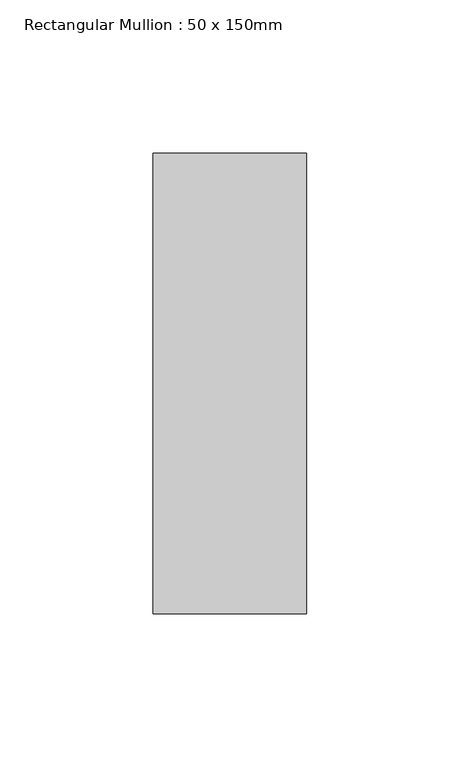
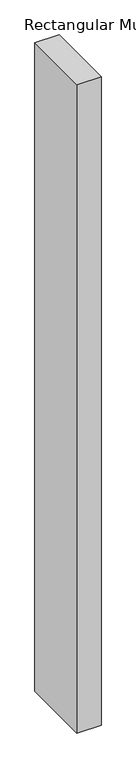
"""IFC4 building model written with IfcOpenShell, lengths in millimetres: member geometry, Rectangular Mullion : 50 x 150mm."""

from ifc_helpers import new_model, si_unit, frame, origin, place, context, project, spatial, polyline, outline, extrude, source, transform, mapped, element, save


def rectangular_mullion_50_x_150mm_695a1f45(model_context):
    return source(origin(), model_context, "Body", "SweptSolid", [
        extrude(outline(polyline([(0.0, 75.0), (0.0, -75.0), (-50.0, -75.0), (-50.0, 75.0), (0.0, 75.0)])), frame((0.0, 0.0, -1416.6666668), z_axis=(0.0, 0.0, 1.0), x_axis=(1.0, 0.0, 0.0)), (0.0, 0.0, 1.0), 1416.6666668),
    ])


if __name__ == "__main__":
    model = new_model("IFC4")
    model_context = context("Model", 3, world=origin())
    ifc_project = project(units=[si_unit("LENGTHUNIT", "METRE", prefix="MILLI")], contexts=[model_context])
    site = spatial("IfcSite", under=ifc_project)
    building = spatial("IfcBuilding", under=site)
    placement = place(None, origin())
    rectangular_mullion_50_x_150mm_shape = rectangular_mullion_50_x_150mm_695a1f45(model_context)
    element("IfcMember", 1, ObjectType="Rectangular Mullion : 50 x 150mm", at=placement, inside=building, context=model_context, shape_type="MappedRepresentation", body=[
        mapped(rectangular_mullion_50_x_150mm_shape, transform((0.0, 0.0, 0.0), x_axis=(1.0, 0.0, 0.0), y_axis=(0.0, 1.0, 0.0), z_axis=(0.0, 0.0, 1.0))),
    ])
    save(model, "model.ifc")

# Revit data of these elements
# Type "Rectangular Mullion : 50 x 150mm"
#   built-in parameter 1007304 = 0.492126 (stored number, unit not read)
#   built-in parameter 1007301 = 0.082021 (stored number, unit not read)
#   built-in parameter 1007300 = 0.082021 (stored number, unit not read)
# Element 1 (IfcMember, "Rectangular Mullion : 50 x 150mm")
#   Materials on its faces: "Aluminium"
# Materials
#   "Aluminium": class "Metal", colour RGB 247 247 247, transparency 0, Description = "Aluminium 6061", Cost = 0
